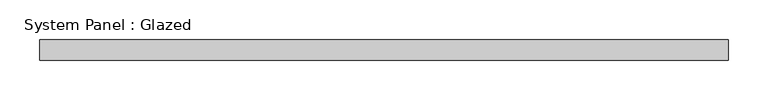
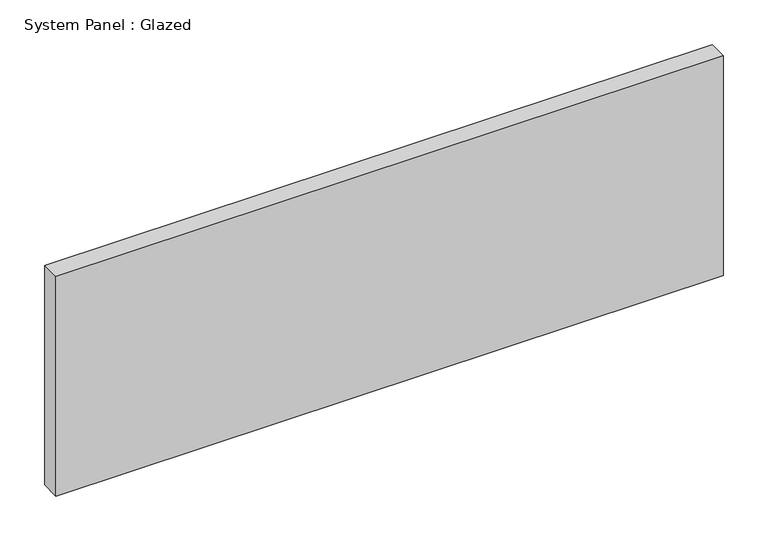
"""IFC4 building model written with IfcOpenShell, lengths in millimetres: plate geometry, System Panel : Glazed."""

from ifc_helpers import new_model, si_unit, origin, origin_with_axes, place, context, project, spatial, polyline, outline, extrude, source, transform, mapped, element, save


def system_panel_glazed_f68cf4a2(model_context):
    return source(origin(), model_context, "Body", "SweptSolid", [
        extrude(outline(polyline([(432.3220098, 19.05), (-432.3220098, 19.05), (-432.3220098, 44.45), (432.3220098, 44.45), (432.3220098, 19.05)])), origin_with_axes(), (0.0, 0.0, 1.0), 300.99),
    ])


if __name__ == "__main__":
    model = new_model("IFC4")
    model_context = context("Model", 3, world=origin())
    ifc_project = project(units=[si_unit("LENGTHUNIT", "METRE", prefix="MILLI")], contexts=[model_context])
    site = spatial("IfcSite", under=ifc_project)
    building = spatial("IfcBuilding", under=site)
    placement = place(None, origin())
    system_panel_glazed_shape = system_panel_glazed_f68cf4a2(model_context)
    element("IfcPlate", 1, ObjectType="System Panel : Glazed", at=placement, inside=building, context=model_context, shape_type="MappedRepresentation", body=[
        mapped(system_panel_glazed_shape, transform((0.0, 0.0, 0.0), x_axis=(1.0, 0.0, 0.0), y_axis=(0.0, 1.0, 0.0), z_axis=(0.0, 0.0, 1.0))),
    ])
    save(model, "model.ifc")

# Revit data of these elements
# Type "System Panel : Glazed"
#   Construction Type Id = "GSP4R"
#   Analytic Construction = "1/8 in Pilkington single glazing"
#   Visual Light Transmittance = 0.9
#   Solar Heat Gain Coefficient = 0.86
#   Heat Transfer Coefficient (U) = 1.18115 BTU/(h·ft²·°F)
#   Define Thermal Properties by = 1
# Element 1 (IfcPlate, "System Panel : Glazed")
#   Materials on its faces: "Glass"
# Materials
#   "Glass": class "Glass", colour RGB 0 128 192, transparency 0.75, Description = "Soda Lime Glass", Cost = 0
